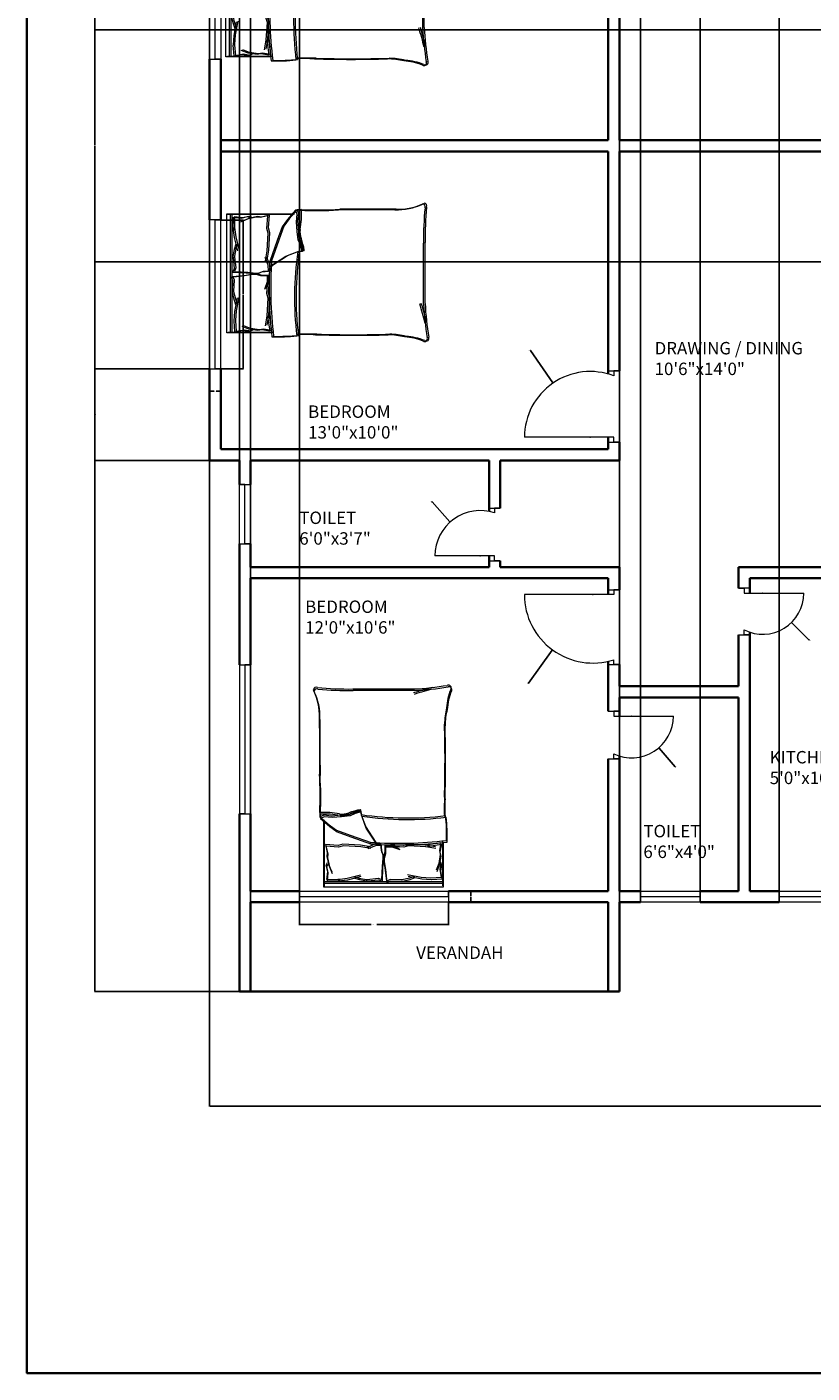
# Model space of a CAD drawing. Units: inches. Extents: x 1937 to 2996, y 1402 to 2323.
# Tile 1 of 10: x 1937 to 2253, y 1402 to 1944. Entities that reach past the tile are written whole.
import ezdxf

# ---------------------------------------------------------------- set-up
doc = ezdxf.new("R2010")
doc.units = ezdxf.units.IN
for name, color, linetype, lineweight in [('A-ANNO-DIMS', 2, 'Continuous', 18), ('A-ANNO-TTLB', 7, 'Continuous', 35), ('A-AREA-IDEN', 7, 'Continuous', 18), ('A-DOOR', 11, 'Continuous', 18), ('A-FURN', 8, 'Continuous', 13), ('A-GLAZ', 141, 'Continuous', 18), ('A-WALL', 7, 'Continuous', 35)]:
    doc.layers.add(name, color=color, linetype=linetype, lineweight=lineweight)
doc.styles.get("Standard").update_dxf_attribs({"font": 'arial.ttf'})
doc.dimstyles.get("Standard").update_dxf_attribs({"dimtxt": 0.18, "dimasz": 0.18, "dimexe": 0.18, "dimexo": 0.0625, "dimgap": 0.09, "dimtad": 0, "dimtih": 1, "dimtoh": 1, "dimdec": 4, "dimzin": 0, "dimdsep": 46, "dimtxsty": 'Standard', "dimcen": 0.09, "dimadec": 0, "dimazin": 0, "dimtfac": 1, "dimtdec": 4, "dimtofl": 0, "dimtmove": 0, "dimatfit": 3, "dimfxl": 1, "dimtolj": 1, "dimtzin": 0, "dimarcsym": 0})

# ---------------------------------------------------------------- blocks, each defined once
blk = doc.blocks.new('BED-DOUBLE')
for p, q in [((-24.01, -18.11), (-24.01, 0)), ((-24.01, -18.11), (-24.01, 0)), ((-24.01, 0), (24.01, 0)), ((23.78, 0), (23.78, -26.61)), ((23.78, 0), (23.78, -26.61)), ((24.01, 0), (24.01, -0.64)), ((-24.01, -1.53), (23.78, -1.53)), ((-24.01, -1.53), (23.78, -1.53)), ((-23.78, -18.75), (-23.78, -0.64)), ((-23.78, -18.75), (-23.78, -0.64)), ((-23.78, -2.17), (24.01, -2.17)), ((-23.78, -2.17), (24.01, -2.17)), ((-23.59, -3.34), (-19.3, -3.01)), ((-23.59, -3.34), (-19.31, -3.01)), ((-23.59, -3.32), (-23.01, -6.5)), ((-23.59, -3.32), (-23.01, -6.5)), ((-23.36, -3.98), (-19.08, -3.65)), ((-23.36, -3.98), (-19.08, -3.65)), ((-23.36, -3.96), (-22.78, -7.14)), ((-23.36, -3.96), (-22.78, -7.14)), ((-19.31, -3.01), (-19.2, -3.03)), ((-19.3, -3.01), (-19.2, -3.03)), ((-19.2, -3.03), (-15.38, -3.32)), ((-19.2, -3.03), (-15.38, -3.32)), ((-19.08, -3.65), (-18.97, -3.67)), ((-19.08, -3.65), (-18.97, -3.67)), ((-18.97, -3.67), (-15.15, -3.96)), ((-18.97, -3.67), (-15.15, -3.96)), ((-15.38, -3.32), (-9.88, -4.33)), ((-15.38, -3.32), (-9.88, -4.33)), ((-15.15, -3.96), (-9.65, -4.97)), ((-15.15, -3.96), (-9.65, -4.97)), ((-12.63, -3.75), (-10.61, -3.03)), ((-12.63, -3.75), (-10.61, -3.03)), ((-12.4, -4.39), (-10.38, -3.67)), ((-12.4, -4.39), (-10.38, -3.67)), ((-10.61, -3.03), (-7.71, -2.3)), ((-10.61, -3.03), (-7.71, -2.3)), ((-10.38, -3.67), (-7.49, -2.94)), ((-10.38, -3.67), (-7.49, -2.94)), ((-7.71, -2.3), (-7.39, -2.3)), ((-7.71, -2.3), (-7.39, -2.3)), ((-7.49, -2.94), (-7.16, -2.94)), ((-7.49, -2.94), (-7.16, -2.94)), ((-7.39, -2.3), (-2.95, -2.45)), ((-7.39, -2.3), (-2.95, -2.45)), ((-7.16, -2.94), (-2.72, -3.09)), ((-7.16, -2.94), (-2.72, -3.09)), ((-2.95, -2.45), (-1.5, -1.87)), ((-2.95, -2.45), (-1.5, -1.87)), ((-2.72, -3.09), (-1.27, -2.51)), ((-2.72, -3.09), (-1.27, -2.51)), ((-1.5, -1.87), (-0.92, -7.22)), ((-1.5, -1.87), (-0.92, -7.22)), ((-1.27, -2.51), (-0.7, -7.86)), ((-1.27, -2.51), (-0.7, -7.86)), ((0.49, -2.49), (0.25, -7.87)), ((0.49, -2.49), (0.25, -7.87)), ((0.72, -3.13), (0.48, -8.51)), ((0.72, -3.13), (0.48, -8.51)), ((1.97, -2.98), (0.49, -2.49)), ((1.97, -2.98), (0.49, -2.49)), ((2.2, -3.62), (0.72, -3.13)), ((2.2, -3.62), (0.72, -3.13)), ((6.4, -2.56), (1.97, -2.98)), ((6.4, -2.56), (1.97, -2.98)), ((6.63, -3.2), (2.2, -3.62)), ((6.63, -3.2), (2.2, -3.62)), ((6.72, -2.54), (6.4, -2.56)), ((6.72, -2.54), (6.4, -2.56)), ((6.95, -3.18), (6.63, -3.2)), ((6.95, -3.18), (6.63, -3.2)), ((9.65, -3.08), (6.72, -2.54)), ((9.65, -3.08), (6.72, -2.54)), ((9.88, -3.72), (6.95, -3.18)), ((9.88, -3.72), (6.95, -3.18)), ((14.43, -3.07), (9.01, -4.42)), ((14.43, -3.07), (9.01, -4.42)), ((14.66, -3.71), (9.24, -5.06)), ((14.66, -3.71), (9.24, -5.06)), ((11.72, -3.67), (9.65, -3.08)), ((11.72, -3.67), (9.65, -3.08)), ((11.94, -4.31), (9.88, -3.72)), ((11.94, -4.31), (9.88, -3.72)), ((18.23, -2.54), (14.43, -3.07)), ((18.23, -2.54), (14.43, -3.07)), ((18.46, -3.18), (14.66, -3.71)), ((18.46, -3.18), (14.66, -3.71)), ((22.63, -2.56), (17.23, -2.46)), ((17.23, -2.46), (18.23, -2.54)), ((22.63, -2.56), (17.23, -2.46)), ((17.23, -2.46), (18.23, -2.54)), ((22.86, -3.2), (17.45, -3.1)), ((17.45, -3.1), (18.46, -3.18)), ((22.86, -3.2), (17.45, -3.1)), ((17.45, -3.1), (18.46, -3.18)), ((22.63, -2.56), (22.25, -5.77)), ((22.63, -2.56), (22.25, -5.77)), ((22.86, -3.2), (22.48, -6.41)), ((22.86, -3.2), (22.48, -6.41)), ((24.01, -0.64), (24.01, -27.25)), ((24.01, -0.64), (24.01, -27.25)), ((-23.01, -6.5), (-23.45, -9.1)), ((-23.01, -6.5), (-23.45, -9.1)), ((-23.45, -9.1), (-22.87, -10.11)), ((-23.45, -9.1), (-22.87, -10.11)), ((-22.78, -7.14), (-23.22, -9.74)), ((-22.78, -7.14), (-23.22, -9.74)), ((-23.22, -9.74), (-22.64, -10.75)), ((-23.22, -9.74), (-22.64, -10.75)), ((-23.01, -12.57), (-22.43, -8.96)), ((-23.01, -12.57), (-22.43, -8.96)), ((-22.78, -13.21), (-22.2, -9.59)), ((-22.78, -13.21), (-22.21, -9.59)), ((-22.43, -8.96), (-21.42, -6.21)), ((-22.43, -8.96), (-21.42, -6.21)), ((-22.21, -9.59), (-21.19, -6.85)), ((-22.2, -9.59), (-21.19, -6.85)), ((-0.92, -7.22), (-0.35, -10.4)), ((-0.92, -7.22), (-0.35, -10.4)), ((-0.7, -7.86), (-0.12, -11.04)), ((-0.7, -7.86), (-0.12, -11.04)), ((-0.35, -10.4), (-0.35, -11.7)), ((-0.35, -10.4), (-0.35, -11.7)), ((0.25, -7.87), (-0.13, -11.08)), ((0.25, -7.87), (-0.13, -11.08)), ((0.48, -8.51), (0.1, -11.72)), ((0.48, -8.51), (0.1, -11.72)), ((21.83, -8.26), (20.64, -5.58)), ((21.82, -8.26), (20.64, -5.58)), ((22.05, -8.9), (20.87, -6.22)), ((22.05, -8.9), (20.87, -6.22)), ((22.63, -11.83), (21.82, -8.26)), ((22.63, -11.83), (21.83, -8.26)), ((22.86, -12.47), (22.05, -8.9)), ((22.86, -12.47), (22.05, -8.9)), ((22.25, -5.77), (22.84, -8.34)), ((22.25, -5.77), (22.84, -8.34)), ((22.84, -8.34), (22.33, -9.38)), ((22.84, -8.34), (22.33, -9.38)), ((22.48, -6.41), (23.07, -8.98)), ((22.48, -6.41), (23.07, -8.98)), ((23.07, -8.98), (22.56, -10.02)), ((23.07, -8.98), (22.56, -10.02)), ((-23.3, -17.34), (-22.72, -14.16)), ((-23.3, -17.34), (-22.72, -14.16)), ((-23.07, -17.98), (-22.49, -14.8)), ((-23.07, -17.98), (-22.49, -14.8)), ((-22.72, -14.16), (-23.01, -12.57)), ((-22.72, -14.16), (-23.01, -12.57)), ((-22.49, -14.8), (-22.78, -13.21)), ((-22.49, -14.8), (-22.78, -13.21)), ((-21.1, -15.63), (-17.07, -16.3)), ((-21.1, -15.63), (-17.07, -16.3)), ((-20.87, -16.27), (-16.84, -16.93)), ((-20.87, -16.27), (-16.84, -16.93)), ((-10.06, -16.73), (-8.1, -16.17)), ((-10.06, -16.73), (-8.1, -16.17)), ((-8.1, -16.17), (-2.97, -16.57)), ((-8.1, -16.17), (-2.97, -16.57)), ((-3.38, -16.26), (-6.53, -15.17)), ((-3.38, -16.26), (-6.53, -15.17)), ((-3.15, -16.9), (-6.3, -15.81)), ((-3.15, -16.9), (-6.3, -15.81)), ((-0.92, -16.26), (-3.38, -16.26)), ((-0.92, -16.26), (-3.38, -16.26)), ((-0.35, -11.7), (-0.92, -13.58)), ((-0.35, -11.7), (-0.92, -13.58)), ((-0.92, -13.58), (-0.92, -16.26)), ((-0.92, -13.58), (-0.92, -16.26)), ((-0.12, -12.34), (-0.7, -14.22)), ((-0.12, -12.34), (-0.7, -14.22)), ((-0.7, -14.22), (-0.7, -16.9)), ((-0.7, -14.22), (-0.7, -16.9)), ((-0.13, -11.08), (-0.05, -12.38)), ((-0.13, -11.08), (-0.05, -12.38)), ((-0.12, -11.04), (-0.12, -12.34)), ((-0.12, -11.04), (-0.12, -12.34)), ((-0.05, -12.38), (0.65, -14.22)), ((-0.05, -12.38), (0.65, -14.22)), ((0.1, -11.72), (0.18, -13.02)), ((0.1, -11.72), (0.18, -13.02)), ((0.18, -13.02), (0.87, -14.86)), ((0.18, -13.02), (0.87, -14.86)), ((0.65, -14.22), (0.81, -16.89)), ((0.65, -14.22), (0.81, -16.89)), ((0.87, -14.86), (1.04, -17.53)), ((0.87, -14.86), (1.04, -17.53)), ((3.27, -16.74), (6.34, -15.45)), ((3.27, -16.74), (6.34, -15.45)), ((3.49, -17.38), (6.56, -16.09)), ((3.49, -17.38), (6.56, -16.09)), ((5.08, -15.63), (9.11, -16.3)), ((5.08, -15.63), (9.11, -16.3)), ((5.31, -16.27), (9.34, -16.93)), ((5.31, -16.27), (9.34, -16.93)), ((16.12, -16.73), (18.08, -16.17)), ((16.12, -16.73), (18.08, -16.17)), ((18.08, -16.17), (23.21, -16.57)), ((18.08, -16.17), (23.21, -16.57)), ((22.44, -13.43), (22.63, -11.83)), ((22.44, -13.43), (22.63, -11.83)), ((23.21, -16.57), (22.44, -13.43)), ((23.21, -16.57), (22.44, -13.43)), ((22.67, -14.07), (22.86, -12.47)), ((22.67, -14.07), (22.86, -12.47)), ((23.44, -17.21), (22.67, -14.07)), ((23.44, -17.21), (22.67, -14.07)), ((-18.2, -16.62), (-23.3, -17.34)), ((-18.2, -16.62), (-23.3, -17.34)), ((-17.98, -17.26), (-23.07, -17.98)), ((-17.98, -17.26), (-23.07, -17.98)), ((-17.07, -16.3), (-18.2, -16.62)), ((-17.07, -16.3), (-18.2, -16.62)), ((-16.84, -16.93), (-17.98, -17.26)), ((-16.84, -16.93), (-17.98, -17.26)), ((-17.07, -16.3), (-10.06, -16.73)), ((-17.07, -16.3), (-10.06, -16.73)), ((-16.84, -16.93), (-9.83, -17.37)), ((-16.84, -16.93), (-9.83, -17.37)), ((-9.83, -17.37), (-7.87, -16.81)), ((-9.83, -17.37), (-7.87, -16.81)), ((-7.87, -16.81), (-2.74, -17.21)), ((-7.87, -16.81), (-2.74, -17.21)), ((-0.7, -16.9), (-3.15, -16.9)), ((-0.7, -16.9), (-3.15, -16.9)), ((0.81, -16.89), (3.27, -16.74)), ((0.81, -16.89), (3.27, -16.74)), ((1.04, -17.53), (3.49, -17.38)), ((1.04, -17.53), (3.49, -17.38)), ((2.77, -17.38), (6.97, -23.88)), ((2.77, -17.38), (6.96, -23.88)), ((3, -18.02), (7.19, -24.52)), ((3, -18.02), (7.19, -24.52)), ((13.16, -20.32), (4.82, -17.38)), ((13.16, -20.32), (4.82, -17.38)), ((13.39, -20.96), (5.05, -18.02)), ((13.39, -20.96), (5.05, -18.02)), ((9.11, -16.3), (16.12, -16.73)), ((9.11, -16.3), (16.12, -16.73)), ((9.34, -16.93), (16.35, -17.37)), ((9.34, -16.93), (16.35, -17.37)), ((18.74, -22.33), (13.16, -20.32)), ((18.74, -22.33), (13.16, -20.32)), ((18.96, -22.97), (13.39, -20.96)), ((18.96, -22.97), (13.39, -20.96)), ((16.35, -17.37), (18.31, -16.81)), ((16.35, -17.37), (18.31, -16.81)), ((18.31, -16.81), (23.44, -17.21)), ((18.31, -16.81), (23.44, -17.21)), ((6.96, -23.88), (8.67, -28.37)), ((6.97, -23.88), (8.67, -28.37)), ((7.19, -24.52), (8.9, -29)), ((7.19, -24.52), (8.9, -29)), ((21.68, -24.5), (18.74, -22.33)), ((21.68, -24.5), (18.74, -22.33)), ((21.91, -25.13), (18.96, -22.97)), ((21.91, -25.13), (18.96, -22.97)), ((25.38, -27.75), (21.68, -24.5)), ((25.38, -27.75), (21.68, -24.5)), ((25.61, -28.39), (21.91, -25.13)), ((25.61, -28.39), (21.91, -25.13)), ((8.67, -28.37), (8.98, -30.38)), ((8.67, -28.37), (8.98, -30.38)), ((8.9, -29), (9.21, -31.02)), ((8.9, -29), (9.21, -31.02)), ((8.98, -30.38), (11.46, -29.76)), ((8.98, -30.38), (11.46, -29.76)), ((9.21, -31.02), (11.68, -30.4)), ((9.21, -31.02), (11.68, -30.4)), ((11.46, -29.76), (13.47, -28.83)), ((11.46, -29.76), (13.47, -28.83)), ((11.68, -30.4), (13.7, -29.47)), ((11.68, -30.4), (13.7, -29.47)), ((13.47, -28.83), (16.88, -28.37)), ((13.47, -28.83), (16.88, -28.37)), ((13.7, -29.47), (17.11, -29)), ((13.7, -29.47), (17.1, -29)), ((16.88, -28.37), (20.75, -28.06)), ((16.88, -28.37), (20.75, -28.06)), ((17.1, -29), (20.98, -28.69)), ((17.11, -29), (20.98, -28.69)), ((20.75, -28.06), (23.85, -28.37)), ((20.75, -28.06), (23.85, -28.37)), ((20.98, -28.69), (24.07, -29)), ((20.98, -28.69), (24.07, -29)), ((23.85, -28.37), (25.38, -27.75)), ((23.85, -28.37), (25.38, -27.75)), ((24.07, -29), (25.61, -28.39)), ((24.07, -29), (25.61, -28.39)), ((25.46, -29.49), (25.38, -27.75, 3.87)), ((25.46, -29.49), (25.38, -27.75, 3.87)), ((25.69, -30.13), (25.61, -28.39, 3.87)), ((25.69, -30.13), (25.61, -28.39, 3.87)), ((-12.42, -79.25), (12.19, -79.25)), ((-12.42, -79.25), (12.19, -79.25)), ((-12.19, -79.88), (12.42, -79.88)), ((-12.19, -79.88), (12.42, -79.88))]:
    blk.add_line(p, q)
for centre, radius, start, end in [((57.68, -20.1), 83.31, 178.7218, 185.604), ((57.68, -20.1), 83.31, 178.7218, 185.604), ((-6.13, -182.05), 164.97, 86.0865, 96.7821), ((-6.13, -182.05), 164.97, 86.0865, 96.7821), ((57.91, -20.74), 83.31, 178.7218, 185.604), ((57.91, -20.74), 83.31, 178.7218, 185.604), ((-5.9, -182.69), 164.97, 86.0865, 96.7821), ((-5.9, -182.69), 164.97, 86.0865, 96.7821), ((-9.73, -156.32), 129.02, 81.7845, 96.9006), ((-9.73, -156.32), 129.02, 81.7845, 96.9006), ((-9.5, -156.96), 129.02, 81.7845, 96.9006), ((-9.5, -156.96), 129.02, 81.7845, 96.9006), ((-194.79, -31.17), 170.11, 358.4762, 1.0082), ((-194.79, -31.17), 170.11, 358.4762, 1.0082), ((-194.56, -31.81), 170.11, 358.4762, 1.0082), ((-194.56, -31.81), 170.11, 358.4762, 1.0082), ((9.15, -30.44), 0.185, 160.2464, 271.1377), ((9.15, -30.44), 0.185, 160.2464, 271.1377), ((3.67, -1.48), 29.65, 280.6617, 289.8806), ((3.67, -1.48), 29.65, 280.6617, 289.8806), ((9.38, -31.08), 0.185, 160.2464, 271.1377), ((9.38, -31.08), 0.185, 160.2464, 271.1377), ((3.9, -2.12), 29.65, 280.6617, 289.8806), ((3.9, -2.12), 29.65, 280.6617, 289.8806), ((16.26, -35.07), 6.22, 78.6608, 113.7384), ((16.26, -35.07), 6.22, 78.6608, 113.7384), ((16.49, -35.71), 6.22, 78.6608, 113.7384), ((16.49, -35.71), 6.22, 78.6608, 113.7384), ((23.84, 6.66), 36.18, 259.8763, 272.5657), ((23.84, 6.66), 36.18, 259.8763, 272.5657), ((24.07, 6.02), 36.18, 259.8763, 272.5657), ((24.07, 6.02), 36.18, 259.8763, 272.5657), ((154.78, -36.32), 129.5, 176.9791, 183.8365), ((154.78, -36.32), 129.5, 176.9791, 183.8365), ((155.01, -36.95), 129.5, 176.9791, 183.8365), ((155.01, -36.95), 129.5, 176.9791, 183.8365), ((457.34, -50.61), 482.31, 178.2277, 181.7185), ((457.34, -50.61), 482.31, 178.2277, 181.7185), ((457.57, -51.25), 482.31, 178.2277, 181.7185), ((457.57, -51.25), 482.31, 178.2277, 181.7185), ((-4536.23, -67.82), 4561.86, 0.00217, 0.28689), ((-4536.23, -67.82), 4561.86, 0.00217, 0.28689), ((-4536, -68.46), 4561.86, 0.00217, 0.28689), ((-4536, -68.46), 4561.86, 0.00217, 0.28689), ((-54.38, -64.52), 29.63, 346.0648, 358.9113), ((-54.38, -64.52), 29.63, 346.0648, 358.9113), ((-54.16, -65.15), 29.63, 346.0648, 358.9113), ((-54.16, -65.15), 29.63, 346.0648, 358.9113), ((48.67, -68.67), 23.07, 177.4714, 206.4681), ((48.67, -68.67), 23.07, 177.4714, 206.4681), ((48.9, -69.31), 23.07, 177.4714, 206.4681), ((48.9, -69.31), 23.07, 177.4714, 206.4681), ((-49.14, -70.28), 23.56, 337.9751, 356.652), ((-49.14, -70.28), 23.56, 337.9751, 356.652), ((-48.92, -70.91), 23.56, 337.9751, 356.652), ((-48.92, -70.91), 23.56, 337.9751, 356.652), ((-26.4, -79.72), 1.09, 146.1736, 293.4781), ((-26.4, -79.72), 1.09, 146.1736, 293.4781), ((-26.17, -80.36), 1.09, 146.1736, 293.4781), ((-26.17, -80.36), 1.09, 146.1736, 293.4781), ((-6.06, -200.84), 121.76, 92.9958, 99.4091), ((-6.06, -200.84), 121.76, 92.9958, 99.4091), ((-5.83, -201.48), 121.76, 92.9958, 99.4091), ((-5.83, -201.48), 121.76, 92.9958, 99.4091), ((-44.71, 23.71), 106.46, 283.3832, 287.7053), ((-44.71, 23.71), 106.46, 283.3832, 287.7053), ((-44.48, 23.07), 106.46, 283.3832, 287.7053), ((-44.48, 23.07), 106.46, 283.3832, 287.7053), ((13.67, -212.28), 133.04, 84.4998, 90.6351), ((13.67, -212.28), 133.04, 84.4998, 90.6351), ((13.9, -212.92), 133.04, 84.4998, 90.6351), ((13.9, -212.92), 133.04, 84.4998, 90.6351), ((26.93, -78.87), 1.1, 242.6588, 356.02), ((26.93, -78.87), 1.1, 242.6588, 356.02), ((27.15, -79.51), 1.1, 242.6588, 356.02), ((27.15, -79.51), 1.1, 242.6588, 356.02)]:
    blk.add_arc(centre, radius, start, end)
blk = doc.blocks.new('WINDOW-60IN')
for p, q in [((0, 2.25), (0, -2.25)), ((0, 2.25), (60, 2.25)), ((0, -2.25), (0, 0)), ((0, 0), (60, 0)), ((60, 0), (60, 2.25)), ((60, 2.25), (60, -2.25)), ((60, -2.25), (0, -2.25))]:
    blk.add_line(p, q)
blk = doc.blocks.new('WINDOW-24IN')
for p, q in [((0, -2.25), (0, 2.25)), ((0, 2.25), (0, 0)), ((24, 2.25), (0, 2.25)), ((0, 0), (24, 0)), ((24, -2.25), (24, 2.25)), ((24, 0), (24, -2.25)), ((0, -2.25), (24, -2.25))]:
    blk.add_line(p, q)
blk = doc.blocks.new('WINDOW-60IN-JAMB-B')
for p, q in [((2.25, 60), (-2.25, 60)), ((-2.25, 60), (-2.25, 0)), ((0, 0), (0, 60)), ((0, 60), (2.25, 60)), ((2.25, 0), (2.25, 60)), ((-2.25, 0), (2.25, 0)), ((2.25, 0), (0, 0))]:
    blk.add_line(p, q)
blk = doc.blocks.new('WINDOW-36IN')
for p, q in [((0, 2.25), (0, -2.25)), ((0, 2.25), (36, 2.25)), ((36, 0), (36, 2.25)), ((36, 2.25), (36, -2.25)), ((0, -2.25), (0, 0)), ((0, 0), (36, 0)), ((36, -2.25), (0, -2.25))]:
    blk.add_line(p, q)
blk = doc.blocks.new('*D11')
at = {"layer": 'A-ANNO-DIMS', "color": 0, "lineweight": -2, "transparency": 16777216}
for p, q in [((2046.82, 1591.24), (2046.82, 1582.13)), ((2106.82, 1591.24), (2106.82, 1582.13)), ((2047, 1582.31), (2075.71, 1582.31)), ((2106.64, 1582.31), (2077.94, 1582.31))]:
    blk.add_line(p, q, dxfattribs=at)
at = {"layer": 'A-ANNO-DIMS', "color": 0, "transparency": 16777216}
for points in [[(2047, 1582.34), (2047, 1582.28), (2046.82, 1582.31)], [(2106.64, 1582.34), (2106.64, 1582.28), (2106.82, 1582.31)]]:
    blk.add_solid(points, dxfattribs=at)
at = {"layer": 'Defpoints', "color": 0, "transparency": 16777216}
for p in [(2046.82, 1591.31), (2106.82, 1591.31), (2106.82, 1582.31)]:
    blk.add_point(p, dxfattribs=at)
at = {"layer": 'A-ANNO-DIMS', "color": 0, "transparency": 16777216, "insert": (2076.82, 1582.31), "char_height": 0.18, "attachment_point": 5}
blk.add_mtext('\\A1;WINDOW 60 TYP.', dxfattribs=at)
blk = doc.blocks.new('*D12')
at = {"layer": 'A-ANNO-DIMS', "color": 0, "lineweight": -2, "transparency": 16777216}
for p, q in [((2106.89, 1595.81), (2116, 1595.81)), ((2115.82, 1595.63), (2115.82, 1593.74)), ((2106.89, 1591.31), (2116, 1591.31)), ((2115.82, 1591.49), (2115.82, 1593.37))]:
    blk.add_line(p, q, dxfattribs=at)
at = {"layer": 'A-ANNO-DIMS', "color": 0, "transparency": 16777216}
for points in [[(2115.79, 1595.63), (2115.85, 1595.63), (2115.82, 1595.81)], [(2115.79, 1591.49), (2115.85, 1591.49), (2115.82, 1591.31)]]:
    blk.add_solid(points, dxfattribs=at)
at = {"layer": 'Defpoints', "color": 0, "transparency": 16777216}
for p in [(2106.82, 1595.81), (2115.82, 1595.81), (2106.82, 1591.31)]:
    blk.add_point(p, dxfattribs=at)
at = {"layer": 'A-ANNO-DIMS', "color": 0, "transparency": 16777216, "insert": (2115.82, 1593.56), "char_height": 0.18, "attachment_point": 5}
blk.add_mtext('\\A1;5 TYP.', dxfattribs=at)
blk = doc.blocks.new('*D19')
at = {"layer": 'A-ANNO-DIMS', "color": 0, "lineweight": -2, "transparency": 16777216}
for p, q in [((2015.21, 1866.15), (2024.33, 1866.15)), ((2024.15, 1865.97), (2024.15, 1836.34)), ((2024.15, 1806.33), (2024.15, 1835.97)), ((2015.21, 1806.15), (2024.33, 1806.15))]:
    blk.add_line(p, q, dxfattribs=at)
at = {"layer": 'A-ANNO-DIMS', "color": 0, "transparency": 16777216}
for points in [[(2024.12, 1865.97), (2024.18, 1865.97), (2024.15, 1866.15)], [(2024.12, 1806.33), (2024.18, 1806.33), (2024.15, 1806.15)]]:
    blk.add_solid(points, dxfattribs=at)
at = {"layer": 'Defpoints', "color": 0, "transparency": 16777216}
for p in [(2015.15, 1866.15), (2024.15, 1866.15), (2015.15, 1806.15)]:
    blk.add_point(p, dxfattribs=at)
at = {"layer": 'A-ANNO-DIMS', "color": 0, "transparency": 16777216, "insert": (2024.15, 1836.15), "char_height": 0.18, "attachment_point": 5}
blk.add_mtext('\\A1;WINDOW B 60 TYP.', dxfattribs=at)
blk = doc.blocks.new('*D20')
at = {"layer": 'A-ANNO-DIMS', "color": 0, "lineweight": -2, "transparency": 16777216}
for p, q in [((2010.65, 1806.09), (2010.65, 1796.97)), ((2015.15, 1806.09), (2015.15, 1796.97)), ((2010.83, 1797.15), (2012.44, 1797.15)), ((2014.97, 1797.15), (2013.36, 1797.15))]:
    blk.add_line(p, q, dxfattribs=at)
at = {"layer": 'A-ANNO-DIMS', "color": 0, "transparency": 16777216}
for points in [[(2010.83, 1797.18), (2010.83, 1797.12), (2010.65, 1797.15)], [(2014.97, 1797.18), (2014.97, 1797.12), (2015.15, 1797.15)]]:
    blk.add_solid(points, dxfattribs=at)
at = {"layer": 'Defpoints', "color": 0, "transparency": 16777216}
for p in [(2010.65, 1806.15), (2015.15, 1806.15), (2015.15, 1797.15)]:
    blk.add_point(p, dxfattribs=at)
at = {"layer": 'A-ANNO-DIMS', "color": 0, "transparency": 16777216, "insert": (2012.9, 1797.15), "char_height": 0.18, "attachment_point": 5}
blk.add_mtext('\\A1;5 TYP.', dxfattribs=at)
blk = doc.blocks.new('*D23')
at = {"layer": 'A-ANNO-DIMS', "color": 0, "lineweight": -2, "transparency": 16777216}
for p, q in [((2010.65, 1769.24), (2010.65, 1508.98)), ((2924.15, 1769.24), (2924.15, 1508.98)), ((2010.83, 1509.16), (2467, 1509.16)), ((2923.97, 1509.16), (2467.79, 1509.16))]:
    blk.add_line(p, q, dxfattribs=at)
at = {"layer": 'A-ANNO-DIMS', "color": 0, "transparency": 16777216}
for points in [[(2010.83, 1509.19), (2010.83, 1509.13), (2010.65, 1509.16)], [(2923.97, 1509.19), (2923.97, 1509.13), (2924.15, 1509.16)]]:
    blk.add_solid(points, dxfattribs=at)
at = {"layer": 'Defpoints', "color": 0, "transparency": 16777216}
for p in [(2010.65, 1769.31), (2924.15, 1769.31), (2924.15, 1509.16)]:
    blk.add_point(p, dxfattribs=at)
at = {"layer": 'A-ANNO-DIMS', "color": 0, "transparency": 16777216, "insert": (2467.4, 1509.16), "char_height": 0.18, "attachment_point": 5}
blk.add_mtext('\\A1;913.5', dxfattribs=at)
blk = doc.blocks.new('*D24')
at = {"layer": 'A-ANNO-DIMS', "color": 0, "lineweight": -2, "transparency": 16777216}
for p, q in [((2022.58, 2236.81), (1964.32, 2236.81)), ((1964.5, 2236.63), (1964.5, 1896.24)), ((1964.5, 1555.49), (1964.5, 1895.87)), ((2022.58, 1555.31), (1964.32, 1555.31))]:
    blk.add_line(p, q, dxfattribs=at)
at = {"layer": 'A-ANNO-DIMS', "color": 0, "transparency": 16777216}
for points in [[(1964.47, 2236.63), (1964.53, 2236.63), (1964.5, 2236.81)], [(1964.47, 1555.49), (1964.53, 1555.49), (1964.5, 1555.31)]]:
    blk.add_solid(points, dxfattribs=at)
at = {"layer": 'Defpoints', "color": 0, "transparency": 16777216}
for p in [(1964.5, 2236.81), (2022.65, 2236.81), (2022.65, 1555.31)]:
    blk.add_point(p, dxfattribs=at)
at = {"layer": 'A-ANNO-DIMS', "color": 0, "transparency": 16777216, "insert": (1964.5, 1896.06), "char_height": 0.18, "attachment_point": 5}
blk.add_mtext('\\A1;681.5', dxfattribs=at)
blk = doc.blocks.new('*D32')
at = {"layer": 'A-ANNO-DIMS', "color": 0, "lineweight": -2, "transparency": 16777216}
for p, q in [((2350.55, 1942.81), (1964.32, 1942.81)), ((1964.5, 1942.63), (1964.5, 1896.24)), ((1964.5, 1849.49), (1964.5, 1895.87)), ((2350.55, 1849.31), (1964.32, 1849.31))]:
    blk.add_line(p, q, dxfattribs=at)
at = {"layer": 'A-ANNO-DIMS', "color": 0, "transparency": 16777216}
for points in [[(1964.47, 1942.63), (1964.53, 1942.63), (1964.5, 1942.81)], [(1964.47, 1849.49), (1964.53, 1849.49), (1964.5, 1849.31)]]:
    blk.add_solid(points, dxfattribs=at)
at = {"layer": 'Defpoints', "color": 0, "transparency": 16777216}
for p in [(1964.5, 1942.81), (2350.61, 1942.81), (2350.61, 1849.31)]:
    blk.add_point(p, dxfattribs=at)
at = {"layer": 'A-ANNO-DIMS', "color": 0, "transparency": 16777216, "insert": (1964.5, 1896.06), "char_height": 0.18, "attachment_point": 5}
blk.add_mtext('\\A1;93.5', dxfattribs=at)
blk = doc.blocks.new('*D44')
at = {"layer": 'A-ANNO-DIMS', "color": 0, "lineweight": -2, "transparency": 16777216}
for p, q in [((2010.65, 1769.37), (2010.65, 2283.14)), ((2022.65, 1769.37), (2022.65, 2283.14)), ((2010.83, 2282.96), (2016.44, 2282.96)), ((2022.47, 2282.96), (2016.86, 2282.96))]:
    blk.add_line(p, q, dxfattribs=at)
at = {"layer": 'A-ANNO-DIMS', "color": 0, "transparency": 16777216}
for points in [[(2010.83, 2282.99), (2010.83, 2282.93), (2010.65, 2282.96)], [(2022.47, 2282.99), (2022.47, 2282.93), (2022.65, 2282.96)]]:
    blk.add_solid(points, dxfattribs=at)
at = {"layer": 'Defpoints', "color": 0, "transparency": 16777216}
for p in [(2022.65, 2282.96), (2010.65, 1769.31), (2022.65, 1769.31)]:
    blk.add_point(p, dxfattribs=at)
at = {"layer": 'A-ANNO-DIMS', "color": 0, "transparency": 16777216, "insert": (2016.65, 2282.96), "char_height": 0.18, "attachment_point": 5}
blk.add_mtext('\\A1;12', dxfattribs=at)
blk = doc.blocks.new('*D45')
at = {"layer": 'A-ANNO-DIMS', "color": 0, "lineweight": -2, "transparency": 16777216}
for p, q in [((2010.58, 1806.15), (1964.32, 1806.15)), ((1964.5, 1805.97), (1964.5, 1787.91)), ((1964.5, 1769.49), (1964.5, 1787.55)), ((2010.58, 1769.31), (1964.32, 1769.31))]:
    blk.add_line(p, q, dxfattribs=at)
at = {"layer": 'A-ANNO-DIMS', "color": 0, "transparency": 16777216}
for points in [[(1964.47, 1805.97), (1964.53, 1805.97), (1964.5, 1806.15)], [(1964.47, 1769.49), (1964.53, 1769.49), (1964.5, 1769.31)]]:
    blk.add_solid(points, dxfattribs=at)
at = {"layer": 'Defpoints', "color": 0, "transparency": 16777216}
for p in [(1964.5, 1806.15), (2010.65, 1806.15), (2010.65, 1769.31)]:
    blk.add_point(p, dxfattribs=at)
at = {"layer": 'A-ANNO-DIMS', "color": 0, "transparency": 16777216, "insert": (1964.5, 1787.73), "char_height": 0.18, "attachment_point": 5}
blk.add_mtext('\\A1;36.846', dxfattribs=at)
blk = doc.blocks.new('*D46')
at = {"layer": 'A-ANNO-DIMS', "color": 0, "lineweight": -2, "transparency": 16777216}
for p, q in [((2027.15, 1591.37), (2027.15, 2283.14)), ((2046.82, 1591.37), (2046.82, 2283.14)), ((2027.33, 2282.96), (2036.53, 2282.96)), ((2046.64, 2282.96), (2037.44, 2282.96))]:
    blk.add_line(p, q, dxfattribs=at)
at = {"layer": 'A-ANNO-DIMS', "color": 0, "transparency": 16777216}
for points in [[(2027.33, 2282.99), (2027.33, 2282.93), (2027.15, 2282.96)], [(2046.64, 2282.99), (2046.64, 2282.93), (2046.82, 2282.96)]]:
    blk.add_solid(points, dxfattribs=at)
at = {"layer": 'Defpoints', "color": 0, "transparency": 16777216}
for p in [(2046.82, 2282.96), (2027.15, 1591.31), (2046.82, 1591.31)]:
    blk.add_point(p, dxfattribs=at)
at = {"layer": 'A-ANNO-DIMS', "color": 0, "transparency": 16777216, "insert": (2036.99, 2282.96), "char_height": 0.18, "attachment_point": 5}
blk.add_mtext('\\A1;19.678', dxfattribs=at)
blk = doc.blocks.new('*D47')
at = {"layer": 'A-ANNO-DIMS', "color": 0, "lineweight": -2, "transparency": 16777216}
for p, q in [((2175.65, 1591.37), (2175.65, 2283.14)), ((2184.14, 1591.37), (2184.14, 2283.14)), ((2175.83, 2282.96), (2179.52, 2282.96)), ((2183.96, 2282.96), (2180.27, 2282.96))]:
    blk.add_line(p, q, dxfattribs=at)
at = {"layer": 'A-ANNO-DIMS', "color": 0, "transparency": 16777216}
for points in [[(2175.83, 2282.99), (2175.83, 2282.93), (2175.65, 2282.96)], [(2183.96, 2282.99), (2183.96, 2282.93), (2184.14, 2282.96)]]:
    blk.add_solid(points, dxfattribs=at)
at = {"layer": 'Defpoints', "color": 0, "transparency": 16777216}
for p in [(2184.14, 2282.96), (2175.65, 1591.31), (2184.14, 1591.31)]:
    blk.add_point(p, dxfattribs=at)
at = {"layer": 'A-ANNO-DIMS', "color": 0, "transparency": 16777216, "insert": (2179.89, 2282.96), "char_height": 0.18, "attachment_point": 5}
blk.add_mtext('\\A1;8.491', dxfattribs=at)
blk = doc.blocks.new('*D48')
at = {"layer": 'A-ANNO-DIMS', "color": 0, "lineweight": -2, "transparency": 16777216}
for p, q in [((2208.14, 1591.37), (2208.14, 2283.14)), ((2239.96, 1591.37), (2239.96, 2283.14)), ((2208.32, 2282.96), (2223.66, 2282.96)), ((2239.78, 2282.96), (2224.44, 2282.96))]:
    blk.add_line(p, q, dxfattribs=at)
at = {"layer": 'A-ANNO-DIMS', "color": 0, "transparency": 16777216}
for points in [[(2208.32, 2282.99), (2208.32, 2282.93), (2208.14, 2282.96)], [(2239.78, 2282.99), (2239.78, 2282.93), (2239.96, 2282.96)]]:
    blk.add_solid(points, dxfattribs=at)
at = {"layer": 'Defpoints', "color": 0, "transparency": 16777216}
for p in [(2239.96, 2282.96), (2208.14, 1591.31), (2239.96, 1591.31)]:
    blk.add_point(p, dxfattribs=at)
at = {"layer": 'A-ANNO-DIMS', "color": 0, "transparency": 16777216, "insert": (2224.05, 2282.96), "char_height": 0.18, "attachment_point": 5}
blk.add_mtext('\\A1;31.82', dxfattribs=at)
blk = doc.blocks.new('*D67')
at = {"layer": 'A-ANNO-DIMS', "color": 0, "lineweight": -2, "transparency": 16777216}
for p, q in [((2164.84, 1715.22), (2165.02, 1715.22)), ((2164.93, 1715.13), (2164.93, 1715.31)), ((2139.01, 1679.6), (2148.62, 1692.81)), ((2138.83, 1679.6), (2139.01, 1679.6))]:
    blk.add_line(p, q, dxfattribs=at)
at = {"layer": 'A-ANNO-DIMS', "color": 0, "transparency": 16777216}
blk.add_solid([(2148.6, 1692.83), (2148.65, 1692.79), (2148.73, 1692.96)], dxfattribs=at)
at = {"layer": 'Defpoints', "color": 0, "transparency": 16777216}
for p in [(2164.93, 1715.22), (2148.73, 1692.96)]:
    blk.add_point(p, dxfattribs=at)
at = {"layer": 'A-ANNO-DIMS', "color": 0, "transparency": 16777216, "insert": (2138.28, 1679.6), "char_height": 0.18, "attachment_point": 5}
blk.add_mtext('\\A1;R27.535', dxfattribs=at)
blk = doc.blocks.new('*D71')
at = {"layer": 'A-ANNO-DIMS', "color": 0, "lineweight": -2, "transparency": 16777216}
for p, q in [((2139.72, 1813.56), (2139.9, 1813.56)), ((2139.9, 1813.56), (2148.79, 1800.6)), ((2163.79, 1778.62), (2163.97, 1778.62)), ((2163.88, 1778.53), (2163.88, 1778.71))]:
    blk.add_line(p, q, dxfattribs=at)
at = {"layer": 'A-ANNO-DIMS', "color": 0, "transparency": 16777216}
blk.add_solid([(2148.81, 1800.62), (2148.76, 1800.59), (2148.89, 1800.46)], dxfattribs=at)
at = {"layer": 'Defpoints', "color": 0, "transparency": 16777216}
for p in [(2148.89, 1800.46), (2163.88, 1778.62)]:
    blk.add_point(p, dxfattribs=at)
at = {"layer": 'A-ANNO-DIMS', "color": 0, "transparency": 16777216, "insert": (2139.17, 1813.56), "char_height": 0.18, "attachment_point": 5}
blk.add_mtext('\\A1;R26.485', dxfattribs=at)
blk = doc.blocks.new('*D81')
at = {"layer": 'A-ANNO-DIMS', "color": 0, "lineweight": -2, "transparency": 16777216}
for p, q in [((2100.04, 1752.61), (2100.22, 1752.61)), ((2100.22, 1752.61), (2107.36, 1744.6)), ((2119.49, 1730.89), (2119.67, 1730.89)), ((2119.58, 1730.8), (2119.58, 1730.98))]:
    blk.add_line(p, q, dxfattribs=at)
at = {"layer": 'A-ANNO-DIMS', "color": 0, "transparency": 16777216}
blk.add_solid([(2107.38, 1744.62), (2107.34, 1744.58), (2107.48, 1744.46)], dxfattribs=at)
at = {"layer": 'Defpoints', "color": 0, "transparency": 16777216}
for p in [(2107.48, 1744.46), (2119.58, 1730.89)]:
    blk.add_point(p, dxfattribs=at)
at = {"layer": 'A-ANNO-DIMS', "color": 0, "transparency": 16777216, "insert": (2099.49, 1752.61), "char_height": 0.18, "attachment_point": 5}
blk.add_mtext('\\A1;R18.184', dxfattribs=at)
blk = doc.blocks.new('*D82')
at = {"layer": 'A-ANNO-DIMS', "color": 0, "lineweight": -2, "transparency": 16777216}
for p, q in [((2180.5, 1666.31), (2180.68, 1666.31)), ((2180.59, 1666.22), (2180.59, 1666.4)), ((2198.1, 1645.89), (2191.65, 1653.41)), ((2198.28, 1645.89), (2198.1, 1645.89))]:
    blk.add_line(p, q, dxfattribs=at)
at = {"layer": 'A-ANNO-DIMS', "color": 0, "transparency": 16777216}
blk.add_solid([(2191.67, 1653.43), (2191.62, 1653.39), (2191.53, 1653.55)], dxfattribs=at)
at = {"layer": 'Defpoints', "color": 0, "transparency": 16777216}
for p in [(2180.59, 1666.31), (2191.53, 1653.55)]:
    blk.add_point(p, dxfattribs=at)
at = {"layer": 'A-ANNO-DIMS', "color": 0, "transparency": 16777216, "insert": (2198.74, 1645.89), "char_height": 0.18, "attachment_point": 5}
blk.add_mtext('\\A1;R16.81', dxfattribs=at)
blk = doc.blocks.new('*D83')
at = {"layer": 'A-ANNO-DIMS', "color": 0, "lineweight": -2, "transparency": 16777216}
for p, q in [((2233.26, 1715.8), (2233.44, 1715.8)), ((2233.35, 1715.71), (2233.35, 1715.89)), ((2251.95, 1696.96), (2245.1, 1703.9)), ((2252.13, 1696.96), (2251.95, 1696.96))]:
    blk.add_line(p, q, dxfattribs=at)
at = {"layer": 'A-ANNO-DIMS', "color": 0, "transparency": 16777216}
blk.add_solid([(2245.12, 1703.92), (2245.08, 1703.88), (2244.98, 1704.02)], dxfattribs=at)
at = {"layer": 'Defpoints', "color": 0, "transparency": 16777216}
for p in [(2233.35, 1715.8), (2244.98, 1704.02)]:
    blk.add_point(p, dxfattribs=at)
at = {"layer": 'A-ANNO-DIMS', "color": 0, "transparency": 16777216, "insert": (2252.61, 1696.96), "char_height": 0.18, "attachment_point": 5}
blk.add_mtext('\\A1;R16.55', dxfattribs=at)

msp = doc.modelspace()

# ---------------------------------------------------------------- linework, layer by layer
at = {"layer": 'A-ANNO-TTLB'}
msp.add_lwpolyline([(1937.1125, 2323.2883), (2995.8132, 2323.2883), (2995.8132, 1401.6335), (1937.1125, 1401.6335)], close=True, dxfattribs=at)
at = {"layer": 'A-DOOR'}
for p, q in [((2171.1473, 1805.3386), (2175.6473, 1805.3386)), ((2175.6473, 1805.3386), (2173.3973, 1805.3386)), ((2173.3973, 1805.3386), (2173.3973, 1803.3386)), ((2173.3973, 1778.6211), (2137.3973, 1778.6211)), ((2171.1473, 1776.6211), (2175.6473, 1776.6211)), ((2173.3973, 1776.6211), (2173.3973, 1778.6211)), ((2175.6473, 1776.6211), (2173.3973, 1776.6211)), ((2123.1473, 1750.1197), (2127.6473, 1750.1197)), ((2127.6473, 1750.1197), (2125.3973, 1750.1197)), ((2125.3973, 1750.1197), (2125.3973, 1748.1197)), ((2125.3973, 1730.8903), (2101.3973, 1730.8903)), ((2125.3973, 1728.8903), (2125.3973, 1730.8903)), ((2123.1473, 1728.8903), (2127.6473, 1728.8903)), ((2127.6473, 1728.8903), (2125.3973, 1728.8903)), ((2173.3973, 1715.2182), (2137.3973, 1715.2182)), ((2171.1473, 1717.2182), (2175.6473, 1717.2182)), ((2175.6473, 1717.2182), (2173.3973, 1717.2182)), ((2173.3973, 1717.2182), (2173.3973, 1715.2182)), ((2228.1473, 1717.8), (2223.6473, 1717.8)), ((2223.6473, 1717.8), (2225.8973, 1717.8)), ((2225.8973, 1717.8), (2225.8973, 1715.8)), ((2225.8973, 1715.8), (2249.8973, 1715.8)), ((2223.6473, 1699.0242), (2228.1473, 1699.0242)), ((2225.8973, 1699.0242), (2225.8973, 1701.0242)), ((2228.1473, 1699.0242), (2225.8973, 1699.0242)), ((2171.1473, 1687.0169), (2175.6473, 1687.0169)), ((2173.3973, 1687.0169), (2173.3973, 1689.0169)), ((2175.6473, 1687.0169), (2173.3973, 1687.0169)), ((2171.1473, 1668.309), (2175.6473, 1668.309)), ((2175.6473, 1668.309), (2173.3973, 1668.309)), ((2173.3973, 1668.309), (2173.3973, 1666.309)), ((2173.3973, 1666.309), (2197.3973, 1666.309)), ((2171.1473, 1649.1135), (2175.6473, 1649.1135)), ((2173.3973, 1649.1135), (2173.3973, 1651.1135)), ((2175.6473, 1649.1135), (2173.3973, 1649.1135))]:
    msp.add_line(p, q, dxfattribs=at)
for centre, radius, start, end in [((2163.8828, 1778.6211), 26.4855, 68.946777, 180), ((2119.5817, 1730.8903), 18.1844, 71.348501, 180), ((2164.9322, 1715.2182), 27.5349, 180, 287.904515), ((2233.3489, 1715.8), 16.5484, 243.237787, 0), ((2180.5868, 1666.309), 16.8105, 244.679612, 360)]:
    msp.add_arc(centre, radius, start, end, dxfattribs=at)
at = {"layer": 'A-WALL'}
for p, q in [((2171.1473, 1986.1318), (2171.1473, 1898.3061)), ((2175.6473, 1984.7551), (2175.6473, 1898.3061)), ((2010.6473, 1930.9695), (2010.6473, 1866.1521)), ((2015.1473, 1930.9695), (2015.1473, 1866.1521)), ((2015.1473, 1898.3061), (2171.1473, 1898.3061)), ((2175.6473, 1898.3061), (2288.1473, 1898.3061)), ((2015.1473, 1893.8061), (2171.1473, 1893.8061)), ((2171.1473, 1893.8061), (2171.1473, 1804.0908)), ((2175.6473, 1893.8061), (2288.1473, 1893.8061)), ((2175.6473, 1893.8061), (2175.6473, 1805.3386)), ((2010.6473, 1806.1521), (2010.6473, 1769.3061)), ((2015.1473, 1806.1521), (2015.1473, 1773.8061)), ((2015.1473, 1773.8061), (2171.1473, 1773.8061)), ((2171.1473, 1778.6211), (2171.1473, 1773.8061)), ((2175.6473, 1776.6211), (2175.6473, 1769.3061)), ((2010.6473, 1769.3061), (2022.6473, 1769.3061)), ((2022.6473, 1769.3061), (2022.6473, 1759.646)), ((2027.1473, 1769.3061), (2027.1473, 1759.646)), ((2027.1473, 1769.3061), (2123.1473, 1769.3061)), ((2123.1473, 1769.3061), (2123.1473, 1748.7217)), ((2127.6473, 1769.3061), (2127.6473, 1750.1197)), ((2127.6473, 1769.3061), (2175.6473, 1769.3061)), ((2022.6473, 1735.646), (2022.6473, 1686.9737)), ((2027.1473, 1735.646), (2027.1473, 1726.3061)), ((2123.1473, 1730.8903), (2123.1473, 1726.3061)), ((2027.1473, 1726.3061), (2123.1473, 1726.3061)), ((2127.6473, 1728.8903), (2127.6473, 1726.3061)), ((2127.6473, 1726.3061), (2175.6473, 1726.3061)), ((2175.6473, 1726.3061), (2175.6473, 1717.2182)), ((2223.6473, 1726.3061), (2223.6473, 1717.8)), ((2223.6473, 1726.3061), (2288.1473, 1726.3061)), ((2027.1473, 1721.8061), (2171.1473, 1721.8061)), ((2027.1473, 1721.8061), (2027.1473, 1686.9737)), ((2171.1473, 1721.8061), (2171.1473, 1715.2182)), ((2228.1473, 1721.8061), (2228.1473, 1715.8)), ((2228.1473, 1721.8061), (2288.1473, 1721.8061)), ((2223.6473, 1699.0242), (2223.6473, 1678.3061)), ((2228.1473, 1700.0903), (2228.1473, 1595.8061)), ((2171.1473, 1688.3939), (2171.1473, 1668.309)), ((2175.6473, 1687.0169), (2175.6473, 1678.3061)), ((2175.6473, 1678.3061), (2223.6473, 1678.3061)), ((2175.6473, 1673.8061), (2223.6473, 1673.8061)), ((2175.6473, 1673.8061), (2175.6473, 1666.309)), ((2223.6473, 1673.8061), (2223.6473, 1595.8061)), ((2171.1473, 1649.1135), (2171.1473, 1595.8061)), ((2175.6473, 1650.2406), (2175.6473, 1595.8061)), ((2022.6473, 1626.9737), (2022.6473, 1555.3061)), ((2027.1473, 1626.9737), (2027.1473, 1595.8061)), ((2027.1473, 1595.8061), (2046.8248, 1595.8061)), ((2106.8248, 1595.8061), (2171.1473, 1595.8061)), ((2175.6473, 1595.8061), (2184.1385, 1595.8061)), ((2208.1385, 1595.8061), (2223.6473, 1595.8061)), ((2228.1473, 1595.8061), (2239.9586, 1595.8061)), ((2027.1473, 1591.3061), (2046.8248, 1591.3061)), ((2027.1473, 1591.3061), (2027.1473, 1555.3061)), ((2106.8248, 1591.3061), (2171.1473, 1591.3061)), ((2171.1473, 1591.3061), (2171.1473, 1555.3061)), ((2175.6473, 1591.3061), (2175.6473, 1555.3061)), ((2175.6473, 1591.3061), (2184.1385, 1591.3061)), ((2208.1385, 1591.3061), (2239.9586, 1591.3061)), ((2022.6473, 1555.3061), (2175.6473, 1555.3061))]:
    msp.add_line(p, q, dxfattribs=at)

# ---------------------------------------------------------------- block references
at = {"layer": 'A-FURN'}
for p, rotation in [((2017.1846, 1955.8397), 89.99999983318573), ((2017.527, 1844.668), 89.99999983318573), ((2080.6874, 1597.332), 180)]:
    msp.add_blockref('BED-DOUBLE', p, dxfattribs=dict(at, rotation=rotation))
at = {"layer": 'A-GLAZ', "rotation": 90}
msp.add_blockref('WINDOW-60IN', (2012.8973, 1930.9695), dxfattribs=at)
at = {"layer": 'A-GLAZ'}
for name, p in [('WINDOW-60IN-JAMB-B', (2012.8973, 1806.1521)), ('WINDOW-60IN', (2046.8248, 1593.5561)), ('WINDOW-36IN', (2239.9586, 1593.5561))]:
    msp.add_blockref(name, p, dxfattribs=at)
at = {"layer": 'A-GLAZ', "extrusion": (0, 0, -1), "zscale": -1}
for name, p, rotation in [('WINDOW-24IN', (-2024.8973, 1735.646), 90), ('WINDOW-60IN', (-2024.8973, 1686.9737), 270), ('WINDOW-24IN', (-2184.1385, 1593.5561), 180)]:
    msp.add_blockref(name, p, dxfattribs=dict(at, rotation=rotation))

# ---------------------------------------------------------------- texts
at = {"layer": 'A-AREA-IDEN', "char_height": 5, "attachment_point": 1}
for s, width, insert in [('DRAWING / DINING \\P10\'6"x14\'0"', 261.360561, (2189.8017, 1817.0161)), ('BEDROOM\\P13\'0"x10\'0"', 162.904506, (2050.3146, 1791.4397)), ('TOILET\\P6\'0"x3\'7"', 152.727307, (2046.7573, 1748.6929)), ('BEDROOM\\P12\'0"x10\'6"', 143.961097, (2049.1211, 1712.8565)), ('KITCHEN\\P5\'0"x10\'6"', 139.189927, (2236.1606, 1652.236)), ('TOILET\\P6\'6"x4\'0"', 162.095513, (2185.2848, 1622.4598)), ('VERANDAH', 137.071433, (2093.8146, 1573.4828))]:
    msp.add_mtext_dynamic_manual_height_columns(s, width=width, gutter_width=12.5, heights=[0], dxfattribs=dict(at, insert=insert))

# ---------------------------------------------------------------- dimensions: what is measured, and where the dimension line sits
at = {"layer": 'A-ANNO-DIMS'}
for base, p1, p2, override, picture, middle in [((2022.6473, 2282.9561), (2010.6473, 1769.3061), (2022.6473, 1769.3061), {"dimdec": 0, "dimlfac": 1, "dimrnd": 0, "dimzin": 0, "dimdsep": 46, "dimlunit": 2}, '*D44', (2016.6473, 2282.9561)), ((2046.82483, 2282.95612), (2027.14731, 1591.30612), (2046.82483, 1591.30612), {"dimdec": 3, "dimlfac": 1, "dimrnd": 0, "dimzin": 0, "dimdsep": 46, "dimlunit": 2}, '*D46', (2036.98607, 2282.95612)), ((2184.1385, 2282.9561), (2175.6473, 1591.3061), (2184.1385, 1591.3061), {"dimdec": 3, "dimlfac": 1, "dimrnd": 0, "dimzin": 0, "dimdsep": 46, "dimlunit": 2}, '*D47', (2179.8929, 2282.9561)), ((2239.9586, 2282.9561), (2208.1385, 1591.3061), (2239.9586, 1591.3061), {"dimdec": 2, "dimlfac": 1, "dimrnd": 0, "dimzin": 0, "dimdsep": 46, "dimlunit": 2}, '*D48', (2224.0486, 2282.9561)), ((2924.1473, 1509.1561), (2010.6473, 1769.3061), (2924.1473, 1769.3061), {"dimdec": 1, "dimlfac": 1, "dimrnd": 0, "dimzin": 0, "dimdsep": 46, "dimlunit": 2}, '*D23', (2467.3973, 1509.1561))]:
    dim = msp.add_linear_dim(base=base, p1=p1, p2=p2, dimstyle='Standard', override=override, dxfattribs=at)
    dim.commit()
    dim.dimension.update_dxf_attribs({"geometry": picture, "text_midpoint": middle})
for base, p1, p2, override, picture, middle in [((1964.4973, 2236.8061), (2022.6473, 1555.3061), (2022.6473, 2236.8061), {"dimdec": 1, "dimlfac": 1, "dimrnd": 0, "dimzin": 0, "dimdsep": 46, "dimlunit": 2}, '*D24', (1964.4973, 1896.0561)), ((1964.4973, 1942.8061), (2350.6104, 1849.3061), (2350.6104, 1942.8061), {"dimdec": 1, "dimlfac": 1, "dimrnd": 0, "dimzin": 0, "dimdsep": 46, "dimlunit": 2}, '*D32', (1964.4973, 1896.0561)), ((1964.4973, 1806.1521), (2010.6473, 1769.3061), (2010.6473, 1806.1521), {"dimdec": 3, "dimlfac": 1, "dimrnd": 0, "dimzin": 0, "dimdsep": 46, "dimlunit": 2}, '*D45', (1964.4973, 1787.7291))]:
    dim = msp.add_linear_dim(base=base, p1=p1, p2=p2, angle=90, dimstyle='Standard', override=override, dxfattribs=at)
    dim.commit()
    dim.dimension.update_dxf_attribs({"geometry": picture, "text_midpoint": middle})
for base, p1, p2, text, picture, middle in [((2024.1473, 1866.1521), (2015.1473, 1806.1521), (2015.1473, 1866.1521), 'WINDOW B <> TYP.', '*D19', (2024.1473, 1836.1521)), ((2115.824828521, 1595.8061190364), (2106.824828521, 1591.3061190364), (2106.824828521, 1595.8061190364), '<> TYP.', '*D12', (2115.824828521, 1593.5561190364))]:
    dim = msp.add_linear_dim(base=base, p1=p1, p2=p2, angle=90, text=text, dimstyle='Standard', override={"dimdec": 0, "dimlfac": 1, "dimrnd": 0, "dimzin": 0, "dimdsep": 46, "dimlunit": 2}, dxfattribs=at)
    dim.commit()
    dim.dimension.update_dxf_attribs({"geometry": picture, "text_midpoint": middle})
for center, mpoint, override, picture, middle in [((2163.8828, 1778.6211), (2148.8909, 1800.4551), {"dimdec": 3, "dimlfac": 1, "dimrnd": 0, "dimzin": 0, "dimdsep": 46, "dimlunit": 2}, '*D71', (2139.1654, 1813.5555)), ((2119.5817, 1730.8903), (2107.4793, 1744.4625), {"dimdec": 3, "dimlfac": 1, "dimrnd": 0, "dimzin": 0, "dimdsep": 46, "dimlunit": 2}, '*D81', (2099.4884, 1752.6058)), ((2164.9322, 1715.2182), (2148.7288, 1692.9557), {"dimdec": 3, "dimlfac": 1, "dimrnd": 0, "dimzin": 0, "dimdsep": 46, "dimlunit": 2}, '*D67', (2138.2763, 1679.5982)), ((2233.3489, 1715.8), (2244.9759, 1704.0244), {"dimdec": 2, "dimlfac": 1, "dimrnd": 0, "dimzin": 0, "dimdsep": 46, "dimlunit": 2}, '*D83', (2252.6126, 1696.9591)), ((2180.5868, 1666.309), (2191.53, 1653.5481), {"dimdec": 2, "dimlfac": 1, "dimrnd": 0, "dimzin": 0, "dimdsep": 46, "dimlunit": 2}, '*D82', (2198.7383, 1645.8916))]:
    dim = msp.add_radius_dim(center=center, mpoint=mpoint, dimstyle='Standard', override=override, dxfattribs=at)
    dim.commit()
    dim.dimension.update_dxf_attribs({"geometry": picture, "text_midpoint": middle, "dimtype": 164})
for base, p1, p2, text, picture, middle in [((2015.1473123667, 1797.1521365884), (2010.6473123667, 1806.1521365884), (2015.1473123667, 1806.1521365884), '<> TYP.', '*D20', (2012.8973123667, 1797.1521365884)), ((2106.8248, 1582.3061), (2046.8248, 1591.3061), (2106.8248, 1591.3061), 'WINDOW <> TYP.', '*D11', (2076.8248, 1582.3061))]:
    dim = msp.add_linear_dim(base=base, p1=p1, p2=p2, text=text, dimstyle='Standard', override={"dimdec": 0, "dimlfac": 1, "dimrnd": 0, "dimzin": 0, "dimdsep": 46, "dimlunit": 2}, dxfattribs=at)
    dim.commit()
    dim.dimension.update_dxf_attribs({"geometry": picture, "text_midpoint": middle})

doc.saveas('drawing.dxf')
